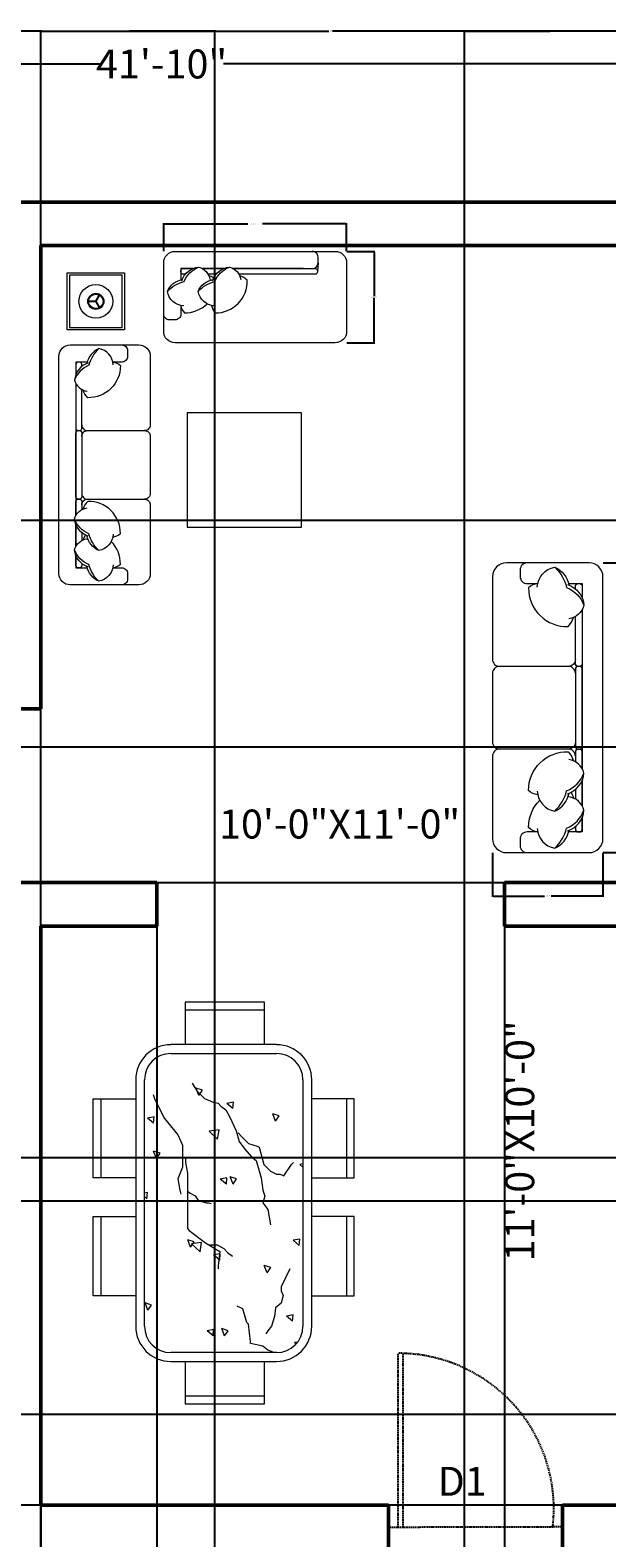
# Model space of a CAD drawing. Units: inches. Extents: x 3 to 576, y -689 to 51.
# Tile 18 of 21: x 262 to 381, y -261 to 51. Entities that reach past the tile are written whole.
import ezdxf

# ---------------------------------------------------------------- set-up
doc = ezdxf.new("R2010")
doc.units = ezdxf.units.IN
doc.header["$MEASUREMENT"] = 0
doc.linetypes.add('DASHED2', pattern=[0.375, 0.25, -0.125])
for name, color, linetype, lineweight in [('A-ANNO-DIMS', 2, 'Continuous', 18), ('A-ANNO-TEXT', 3, 'Continuous', 18), ('A-AREA-IDEN', 7, 'Continuous', 18), ('A-DOOR', 4, 'DASHED2', 25), ('A-FURN', 8, 'Continuous', 18), ('A-WALL', 7, 'Continuous', 50)]:
    doc.layers.add(name, color=color, linetype=linetype, lineweight=lineweight)
doc.styles.get("Standard").update_dxf_attribs({"font": 'arial.ttf'})
doc.dimstyles.get("Standard").update_dxf_attribs({"dimtxt": 0.18, "dimasz": 0.18, "dimexe": 0.18, "dimexo": 0.0625, "dimgap": 0.09, "dimtad": 0, "dimtih": 1, "dimtoh": 1, "dimdec": 0, "dimzin": 0, "dimdsep": 46, "dimlunit": 3, "dimtxsty": 'Standard', "dimcen": 0.09, "dimadec": 0, "dimazin": 0, "dimtfac": 1, "dimtdec": 0, "dimtofl": 0, "dimtmove": 0, "dimatfit": 3, "dimfxl": 1, "dimtolj": 1, "dimtzin": 0, "dimarcsym": 0})

# ---------------------------------------------------------------- blocks, each defined once
blk = doc.blocks.new('*D1')
at = {"layer": 'A-ANNO-DIMS', "color": 0, "lineweight": -2, "transparency": 16777216}
for p, q in [((38.29, 15.75), (38.29, 44.49)), ((38.47, 44.31), (276.45, 44.31)), ((540.11, 44.31), (302.14, 44.31)), ((540.29, 15.75), (540.29, 44.49))]:
    blk.add_line(p, q, dxfattribs=at)
at = {"layer": 'A-ANNO-DIMS', "color": 0, "transparency": 16777216}
for points in [[(38.47, 44.34), (38.47, 44.28), (38.29, 44.31)], [(540.11, 44.34), (540.11, 44.28), (540.29, 44.31)]]:
    blk.add_solid(points, dxfattribs=at)
at = {"layer": 'Defpoints', "color": 0, "transparency": 16777216}
for p in [(540.29, 44.31), (38.29, 15.69), (540.29, 15.69)]:
    blk.add_point(p, dxfattribs=at)
at = {"layer": 'A-ANNO-DIMS', "color": 0, "transparency": 16777216, "insert": (289.29, 44.31), "char_height": 6, "attachment_point": 5}
blk.add_mtext('\\A1;41\'-10"', dxfattribs=at)
blk = doc.blocks.new('DAY BED1')
at = {"color": 0}
blk.add_line((0.3, 0.25), (0.225, 0.255), dxfattribs=at)
blk.add_lwpolyline([(-0.3, 0, -0.414214), (-0.4, 0.1), (-0.4, 0.1, 0.317837), (-0.4, 0.1, -0.414214), (-0.4, 0.1), (-0.4, 0.1, 1.186185), (-0.4, 0.1, -0.414214), (-0.4, 0.1), (-0.4, 1.5, -0.414214), (-0.3, 1.6), (0.3, 1.6, -0.414214), (0.4, 1.5), (0.4, 0.1, -0.414214), (0.3, 0)], format="xyb", close=True, dxfattribs=at)
for points in [[(-0.073, 1.45), (-0.15, 1.45, -0.414214), (-0.2, 1.5), (-0.2, 1.55, -0.414214), (-0.15, 1.6)], [(-0.076, 1.425, -0.356772), (0.05, 1.568, -0.249542), (0.154, 1.438, 9.61688)], [(0.05, 1.568, -0.14773), (0.136, 1.422, -0.213343), (0.262, 1.293, -0.178662)], [(-0.073, 1.45, 0.165541), (-0.139, 1.419, 0.200231), (-0.058, 1.221, 0.121523)], [(0.143, 1.442, -0.306663), (0.262, 1.293, -0.30633), (0.154, 1.196, 0.872847)], [(0.25, 1.345), (0.25, 1.45), (0.152, 1.45, -0.414214)], [(0.2, 1.412), (0.2, 1.43, -0.414214), (0.22, 1.45), (0.23, 1.45, -0.414214), (0.25, 1.43)], [(0.25, 1.43), (0.25, 1.345, -0.414214)], [(-0.076, 1.156, -0.356772), (0.05, 1.299, -0.249542), (0.154, 1.169, 9.61688)], [(0.05, 1.299, -0.14773), (0.136, 1.153, -0.213343), (0.262, 1.024, -0.178662)], [(0.168, 1.163, 0.071865), (0.187, 1.205, -7.115464)], [(0.2, 1.142), (0.2, 1.211, -0.414214)], [(0.25, 1.262), (0.25, 1.075, -0.414214)], [(-0.073, 1.181, 0.165541), (-0.139, 1.15, 0.425989), (0.148, 0.869, 0.121523), (0.187, 0.936, -7.115464)], [(0.143, 1.173, -0.306663), (0.262, 1.024, -0.30633), (0.154, 0.926, 0.872847)], [(0.25, 0.992), (0.25, 0.275, -0.414214), (0.23, 0.255), (0.22, 0.255, -0.414214), (0.2, 0.275), (0.2, 0.942, -0.414214)], [(0.25, 0.377), (0.25, 0.3, 0.414214), (0.3, 0.25), (0.35, 0.25, 0.414214), (0.4, 0.3)]]:
    blk.add_lwpolyline(points, format="xyb", dxfattribs=at)
for points in [[(0.25, 1.075), (0.25, 1.262)], [(0.25, 0.377), (0.25, 0.992)]]:
    blk.add_lwpolyline(points, dxfattribs=at)
blk = doc.blocks.new('DINING-SET-6')
for p, q in [((35.44, 83.21), (19.03, 83.21)), ((19.03, 83.21), (19.03, 74.43)), ((19.03, 81.61), (35.44, 81.61)), ((35.44, 74.43), (35.44, 83.21)), ((37.96, 74.43), (16.08, 74.43)), ((16.08, 72.6), (37.96, 72.6)), ((8.79, 67.13), (8.79, 16.08)), ((10.61, 16.08), (10.61, 67.13)), ((20.49, 66.46), (21.48, 64.87)), ((43.43, 67.13), (43.43, 16.08)), ((45.25, 16.08), (45.25, 67.13)), ((0, 46.82), (0, 63.23)), ((0, 63.23), (8.79, 63.23)), ((1.6, 63.23), (1.6, 46.82)), ((12.38, 64.08), (12.77, 63.09)), ((12.77, 63.09), (14.75, 59.12)), ((21.9, 63.9), (21.31, 65.43)), ((22.64, 64.98), (21.31, 65.43)), ((21.48, 64.87), (23.07, 63.29)), ((21.9, 63.9), (22.63, 64.98)), ((23.07, 63.29), (24.85, 62.49)), ((24.85, 62.49), (25.84, 62.3)), ((29.06, 62.49), (27.69, 62.24)), ((28.94, 61.18), (29.06, 62.49)), ((54.04, 63.23), (45.25, 63.23)), ((52.44, 63.23), (52.44, 46.82)), ((54.04, 46.82), (54.04, 63.23)), ((12.6, 59.46), (11.23, 59.2)), ((12.49, 58.15), (12.6, 59.46)), ((25.84, 62.3), (26.44, 61.7)), ((26.44, 61.7), (27.43, 60.91)), ((27.43, 60.91), (28.22, 59.52)), ((28.94, 61.18), (27.69, 62.24)), ((28.22, 59.52), (29.6, 56.55)), ((38.5, 59.66), (37.18, 60.1)), ((37.77, 58.57), (37.18, 60.1)), ((37.77, 58.57), (38.5, 59.66)), ((12.49, 58.15), (11.23, 59.2)), ((14.75, 59.12), (17.52, 55.75)), ((26.06, 56.77), (23.98, 56.52)), ((25.76, 54.82), (23.98, 56.52)), ((25.76, 54.82), (26.06, 56.77)), ((29.6, 56.55), (30.2, 54.36)), ((17.52, 55.75), (18.51, 53.57)), ((18.51, 53.57), (18.51, 49.01)), ((30, 56.15), (30.79, 55.36)), ((30.2, 54.36), (31.39, 52.78)), ((30.79, 55.36), (32.18, 53.97)), ((32.18, 53.97), (33.96, 53.37)), ((33.96, 53.37), (34.36, 53.18)), ((34.36, 53.18), (35.35, 49.61)), ((13.09, 50.84), (12.5, 52.37)), ((13.83, 51.93), (12.5, 52.37)), ((13.09, 50.84), (13.83, 51.92)), ((19.11, 51.19), (19.11, 50)), ((19.11, 50), (19.5, 47.82)), ((31.39, 52.78), (32.77, 51.19)), ((32.77, 51.19), (33.76, 50.4)), ((33.76, 50.4), (34.75, 46.83)), ((41.09, 49.61), (41.49, 50)), ((18.51, 49.01), (17.52, 46.63)), ((19.5, 47.82), (19.5, 36.32)), ((28.96, 45.51), (28.37, 47.05)), ((29.69, 46.6), (28.37, 47.05)), ((35.35, 49.61), (36.73, 48.22)), ((36.73, 48.22), (37.92, 47.62)), ((37.92, 47.62), (38.71, 47.62)), ((38.71, 47.62), (39.5, 47.23)), ((39.5, 47.23), (41.09, 49.61)), ((43.43, 49.7), (42.77, 49.58)), ((43.43, 49.03), (42.77, 49.58)), ((8.79, 46.82), (0, 46.82)), ((11.23, 43.76), (10.61, 43.65)), ((11.11, 42.46), (11.23, 43.76)), ((17.52, 46.63), (17.92, 44.25)), ((17.92, 44.25), (18.12, 43.46)), ((19.5, 44.06), (20.09, 43.66)), ((27.69, 46.8), (26.31, 46.55)), ((27.57, 45.49), (26.31, 46.55)), ((27.57, 45.49), (27.68, 46.8)), ((28.96, 45.51), (29.69, 46.6)), ((34.75, 46.83), (35.15, 44.25)), ((35.15, 44.25), (35.54, 43.06)), ((45.25, 46.82), (54.04, 46.82)), ((11.11, 42.46), (10.61, 42.88)), ((20.09, 43.66), (21.08, 43.07)), ((21.08, 43.07), (21.68, 42.27)), ((21.68, 42.27), (22.67, 41.88)), ((22.67, 41.88), (23.46, 41.68)), ((23.46, 41.68), (23.85, 41.68)), ((23.85, 41.68), (24.45, 41.48)), ((35.54, 43.06), (35.15, 41.68)), ((35.15, 41.68), (36.14, 40.29)), ((0, 22.39), (0, 38.8)), ((0, 38.8), (8.79, 38.8)), ((1.6, 38.8), (1.6, 22.39)), ((36.14, 40.29), (36.73, 37.12)), ((54.04, 38.8), (45.25, 38.8)), ((52.44, 38.8), (52.44, 22.39)), ((54.04, 22.39), (54.04, 38.8)), ((19.5, 36.32), (19.9, 35.93)), ((19.9, 35.93), (23.27, 33.35)), ((20.15, 32.45), (19.56, 33.99)), ((20.88, 33.54), (19.56, 33.99)), ((20.15, 32.45), (20.88, 33.54)), ((22.44, 33.42), (20.36, 33.17)), ((22.14, 31.47), (20.36, 33.17)), ((22.14, 31.47), (22.44, 33.42)), ((23.27, 33.35), (26.24, 31.57)), ((23.86, 32.95), (25.64, 32.95)), ((25.64, 32.95), (27.03, 32.16)), ((26.24, 31.57), (25.84, 28.59)), ((27.03, 32.16), (27.82, 31.37)), ((27.82, 31.37), (28.81, 30.57)), ((42.77, 34.14), (41.4, 33.89)), ((42.65, 32.83), (41.4, 33.89)), ((42.65, 32.83), (42.77, 34.14)), ((26.31, 31.11), (24.94, 30.85)), ((26.2, 29.8), (24.94, 30.85)), ((25.84, 28.59), (25.84, 28)), ((26.2, 29.8), (26.31, 31.11)), ((36.01, 27.13), (35.43, 28.66)), ((36.75, 28.22), (35.43, 28.66)), ((36.01, 27.13), (36.75, 28.22)), ((40.69, 28), (38.9, 24.23)), ((8.79, 22.39), (0, 22.39)), ((38.9, 24.23), (38.9, 23.44)), ((38.9, 23.44), (39.3, 22.45)), ((39.3, 22.45), (38.9, 20.86)), ((45.25, 22.39), (54.04, 22.39)), ((11.34, 19.39), (10.75, 20.93)), ((12.07, 20.48), (10.75, 20.93)), ((11.34, 19.39), (12.07, 20.48)), ((30.99, 19.67), (29.8, 20.27)), ((31.78, 16.89), (30.99, 19.67)), ((37.72, 19.87), (37.52, 18.09)), ((38.9, 20.86), (37.72, 19.87)), ((32.18, 16.5), (31.78, 16.89)), ((32.57, 12.93), (32.18, 16.5)), ((36.92, 16.1), (36.13, 15.11)), ((37.52, 18.09), (36.92, 16.1)), ((41.28, 17.14), (40.02, 18.2)), ((41.4, 18.45), (40.03, 18.2)), ((41.28, 17.14), (41.4, 18.45)), ((24.94, 15.41), (23.57, 15.16)), ((24.82, 14.11), (23.57, 15.16)), ((24.82, 14.11), (24.94, 15.41)), ((27.21, 14.07), (26.62, 15.6)), ((27.94, 15.16), (26.62, 15.6)), ((27.21, 14.07), (27.94, 15.16)), ((32.57, 12.53), (32.57, 12.93)), ((35.15, 11.94), (32.57, 12.53)), ((36.13, 15.11), (35.74, 14.52)), ((42.34, 12.8), (41.67, 12.72)), ((42.01, 12.4), (41.67, 12.72)), ((37.96, 10.61), (16.08, 10.61)), ((36.14, 11.15), (35.15, 11.94)), ((37.13, 10.75), (36.14, 11.15)), ((16.08, 8.79), (37.96, 8.79)), ((19.03, 8.79), (19.03, 0)), ((35.44, 0), (35.44, 8.79)), ((35.44, 1.6), (19.03, 1.6)), ((19.03, 0), (35.44, 0))]:
    blk.add_line(p, q)
for centre, radius, start, end in [((16.08, 67.13), 7.29, 90, 180), ((16.08, 67.13), 5.47, 90, 180), ((37.96, 67.13), 7.29, 0, 90), ((37.96, 67.13), 5.47, 0, 90), ((16.08, 16.08), 7.29, 180, 270), ((16.08, 16.08), 5.47, 180, 270), ((37.96, 16.08), 5.47, 270, 0), ((37.96, 16.08), 7.29, 270, 0)]:
    blk.add_arc(centre, radius, start, end)
blk = doc.blocks.new('SOFA-3SEAT')
at = {"ltscale": 0.03}
blk.add_lwpolyline([(2.86, 60.03, 0.414214), (0, 57.17), (0, 40.02, 0.414214), (1.43, 38.59, 0.414214), (0, 37.16), (0, 22.87, 0.414214), (1.43, 21.44, 0.414214), (0, 20.01), (0, 2.86, 0.414214), (2.86, 0), (20.01, 0, 0.414214), (22.87, 2.86), (22.87, 57.17, 0.414214), (20.01, 60.03)], format="xyb", close=True, dxfattribs=at)
for points in [[(7.15, 60.03, 0.414214), (5.72, 58.6), (5.72, 57.17, 0.414214), (7.15, 55.74), (9.36, 55.74)], [(9.27, 55.02, -0.356772), (12.88, 59.12, -0.249542), (15.84, 55.41, 9.61688)], [(12.88, 59.12, -0.14773), (15.33, 54.94, -0.213343), (18.93, 51.25, -0.178662)], [(9.36, 55.74, 0.165541), (7.47, 54.86, 0.425989), (15.66, 46.83, 0.121523), (16.79, 48.74, -7.115464)], [(15.53, 55.52, -0.306663), (18.93, 51.25, -0.30633), (15.82, 48.47, 0.872847)], [(17.15, 54.65), (17.15, 55.17, -0.414214), (17.72, 55.74), (18.01, 55.74, -0.414214), (18.58, 55.17)], [(18.58, 55.17), (18.58, 52.73, -0.414214)], [(18.58, 50.35), (18.58, 39.16, -0.414214), (18.01, 38.59), (17.72, 38.59, -0.414214), (17.15, 39.16), (17.15, 48.91, -0.414214)], [(17.15, 40.02, -0.414214), (15.72, 38.59), (1.43, 38.59, -0.414214)], [(17.15, 37.16, 0.414214), (15.72, 38.59)], [(17.15, 22.87, -0.414214), (15.72, 21.44)], [(17.15, 20.01, 0.414214), (15.72, 21.44), (1.43, 21.44, 0.414214)], [(9.36, 11.98, -0.165541), (7.47, 12.87, -0.425989), (15.66, 20.89, -0.121523), (16.79, 18.99, 7.115464)], [(15.53, 12.21, 0.306663), (18.93, 16.47, 0.30633), (15.82, 19.26, -0.872847)], [(18.58, 17.37), (18.58, 20.87, 0.414214), (18.01, 21.44), (17.72, 21.44, 0.414214), (17.15, 20.87), (17.15, 18.81, 0.414214)], [(12.88, 8.61, 0.14773), (15.33, 12.79, 0.213343), (18.93, 16.47, 0.178662)], [(9.27, 12.7, 0.356772), (12.88, 8.61, 0.249542), (15.84, 12.32, -9.61688)], [(17.15, 13.08), (17.15, 11.11, 0.414214)], [(18.58, 9.67), (18.58, 14.99, 0.414214)], [(9.36, 4.28, -0.165541), (7.47, 5.17, -0.200231), (9.77, 10.84, -0.121523)], [(15.53, 4.51, 0.306663), (18.93, 8.77, 0.30633), (15.82, 11.56, -0.872847)], [(16.23, 12.49, -0.071865), (16.79, 11.29, 7.115464)], [(12.88, 0.91, 0.14773), (15.33, 5.09, 0.213343), (18.93, 8.77, 0.178662)], [(18.58, 7.29), (18.58, 4.29), (15.77, 4.29, 0.414214)], [(18.58, 4.86), (18.58, 7.29, 0.414214)], [(9.36, 4.29), (7.15, 4.29, 0.414214), (5.72, 2.86), (5.72, 1.43, 0.414214), (7.15, 0)], [(9.27, 5, 0.356772), (12.88, 0.91, 0.249542), (15.84, 4.62, -9.61688)], [(17.15, 5.38), (17.15, 4.86, 0.414214), (17.72, 4.29), (18.01, 4.29, 0.414214), (18.58, 4.86)]]:
    blk.add_lwpolyline(points, format="xyb")
for points in [[(15.77, 55.74), (18.58, 55.74), (18.58, 52.73)], [(18.58, 50.35), (18.58, 17.37)], [(18.58, 14.99), (18.58, 9.67)]]:
    blk.add_lwpolyline(points)
blk.add_lwpolyline([(18.58, 22.01), (18.58, 38.02, 0.414214), (18.01, 38.59), (17.72, 38.59, 0.414214), (17.15, 38.02), (17.15, 22.01, 0.414214), (17.72, 21.44), (18.01, 21.44, 0.414214)], format="xyb", close=True)
blk = doc.blocks.new('DOOR-SWING-900')
for p, q in [((35.95, 36), (35.95, 34)), ((36, 2), (35.95, 34)), ((36, 2), (0, 2)), ((36, 0), (36, 2))]:
    blk.add_line(p, q)
blk.add_arc((32.22, 2), 32.22, 83.347, 180)
blk = doc.blocks.new('*D31')
at = {"layer": 'A-ANNO-DIMS', "color": 0, "lineweight": -2, "transparency": 16777216}
for p, q in [((289.72, 5.54), (289.72, 11.34)), ((289.9, 11.16), (307.16, 11.16)), ((327.42, 11.16), (310.15, 11.16)), ((327.6, 5.54), (327.6, 11.34))]:
    blk.add_line(p, q, dxfattribs=at)
at = {"layer": 'A-ANNO-DIMS', "color": 0, "transparency": 16777216}
for points in [[(289.9, 11.19), (289.9, 11.13), (289.72, 11.16)], [(327.42, 11.19), (327.42, 11.13), (327.6, 11.16)]]:
    blk.add_solid(points, dxfattribs=at)
at = {"layer": 'Defpoints', "color": 0, "transparency": 16777216}
for p in [(289.72, 11.16), (289.72, 5.48), (327.6, 5.48)]:
    blk.add_point(p, dxfattribs=at)
at = {"layer": 'A-ANNO-DIMS', "color": 0, "transparency": 16777216, "insert": (308.66, 11.16), "char_height": 0.18, "attachment_point": 5}
blk.add_mtext('\\A1;2-SEAT SOFA 3\'-2" TYP.', dxfattribs=at)
blk = doc.blocks.new('*D32')
at = {"layer": 'A-ANNO-DIMS', "color": 0, "lineweight": -2, "transparency": 16777216}
for p, q in [((327.66, 5.48), (333.46, 5.48)), ((333.28, 5.3), (333.28, -3.81)), ((333.28, -13.28), (333.28, -4.17)), ((327.66, -13.46), (333.46, -13.46))]:
    blk.add_line(p, q, dxfattribs=at)
at = {"layer": 'A-ANNO-DIMS', "color": 0, "transparency": 16777216}
for points in [[(333.25, 5.3), (333.31, 5.3), (333.28, 5.48)], [(333.25, -13.28), (333.31, -13.28), (333.28, -13.46)]]:
    blk.add_solid(points, dxfattribs=at)
at = {"layer": 'Defpoints', "color": 0, "transparency": 16777216}
for p in [(327.6, 5.48), (333.28, 5.48), (327.6, -13.46)]:
    blk.add_point(p, dxfattribs=at)
at = {"layer": 'A-ANNO-DIMS', "color": 0, "transparency": 16777216, "insert": (333.28, -3.99), "char_height": 0.18, "attachment_point": 5}
blk.add_mtext('\\A1;1\'-7" TYP.', dxfattribs=at)
blk = doc.blocks.new('*D35')
at = {"layer": 'A-ANNO-DIMS', "color": 0, "lineweight": -2, "transparency": 16777216}
for p, q in [((380.75, -59.06), (389.87, -59.06)), ((389.69, -59.24), (389.69, -88.89)), ((389.69, -118.91), (389.69, -89.26)), ((380.75, -119.09), (389.87, -119.09))]:
    blk.add_line(p, q, dxfattribs=at)
at = {"layer": 'A-ANNO-DIMS', "color": 0, "transparency": 16777216}
for points in [[(389.66, -59.24), (389.72, -59.24), (389.69, -59.06)], [(389.66, -118.91), (389.72, -118.91), (389.69, -119.09)]]:
    blk.add_solid(points, dxfattribs=at)
at = {"layer": 'Defpoints', "color": 0, "transparency": 16777216}
for p in [(380.69, -59.06), (389.69, -59.06), (380.69, -119.09)]:
    blk.add_point(p, dxfattribs=at)
at = {"layer": 'A-ANNO-DIMS', "color": 0, "transparency": 16777216, "insert": (389.69, -89.08), "char_height": 0.18, "attachment_point": 5}
blk.add_mtext('\\A1;3-SEAT SOFA 5\'-0" TYP.', dxfattribs=at)
blk = doc.blocks.new('*D36')
at = {"layer": 'A-ANNO-DIMS', "color": 0, "lineweight": -2, "transparency": 16777216}
for p, q in [((357.82, -119.15), (357.82, -128.27)), ((380.69, -119.15), (380.69, -128.27)), ((358, -128.09), (368.55, -128.09)), ((380.51, -128.09), (369.95, -128.09))]:
    blk.add_line(p, q, dxfattribs=at)
at = {"layer": 'A-ANNO-DIMS', "color": 0, "transparency": 16777216}
for points in [[(358, -128.06), (358, -128.12), (357.82, -128.09)], [(380.51, -128.06), (380.51, -128.12), (380.69, -128.09)]]:
    blk.add_solid(points, dxfattribs=at)
at = {"layer": 'Defpoints', "color": 0, "transparency": 16777216}
for p in [(357.82, -119.09), (380.69, -119.09), (380.69, -128.09)]:
    blk.add_point(p, dxfattribs=at)
at = {"layer": 'A-ANNO-DIMS', "color": 0, "transparency": 16777216, "insert": (369.25, -128.09), "char_height": 0.18, "attachment_point": 5}
blk.add_mtext('\\A1;1\'-11" TYP.', dxfattribs=at)
blk = doc.blocks.new('*D43')
at = {"layer": 'A-ANNO-DIMS', "color": 0, "lineweight": -2, "transparency": 16777216}
for p, q in [((255.29, 6.75), (255.29, 51.32)), ((255.47, 51.14), (259.46, 51.14)), ((264.11, 51.14), (260.12, 51.14)), ((264.29, 6.75), (264.29, 51.32))]:
    blk.add_line(p, q, dxfattribs=at)
at = {"layer": 'A-ANNO-DIMS', "color": 0, "transparency": 16777216}
for points in [[(255.47, 51.17), (255.47, 51.11), (255.29, 51.14)], [(264.11, 51.17), (264.11, 51.11), (264.29, 51.14)]]:
    blk.add_solid(points, dxfattribs=at)
at = {"layer": 'Defpoints', "color": 0, "transparency": 16777216}
for p in [(264.29, 51.14), (255.29, 6.69), (264.29, 6.69)]:
    blk.add_point(p, dxfattribs=at)
at = {"layer": 'A-ANNO-DIMS', "color": 0, "transparency": 16777216, "insert": (259.79, 51.14), "char_height": 0.18, "attachment_point": 5}
blk.add_mtext('\\A1;0\'-9"', dxfattribs=at)
blk = doc.blocks.new('*D44')
at = {"layer": 'A-ANNO-DIMS', "color": 0, "lineweight": -2, "transparency": 16777216}
for p, q in [((264.29, 6.75), (264.29, 51.32)), ((264.47, 51.14), (323.9, 51.14)), ((384.11, 51.14), (324.68, 51.14)), ((384.29, 6.75), (384.29, 51.32))]:
    blk.add_line(p, q, dxfattribs=at)
at = {"layer": 'A-ANNO-DIMS', "color": 0, "transparency": 16777216}
for points in [[(264.47, 51.17), (264.47, 51.11), (264.29, 51.14)], [(384.11, 51.17), (384.11, 51.11), (384.29, 51.14)]]:
    blk.add_solid(points, dxfattribs=at)
at = {"layer": 'Defpoints', "color": 0, "transparency": 16777216}
for p in [(384.29, 51.14), (264.29, 6.69), (384.29, 6.69)]:
    blk.add_point(p, dxfattribs=at)
at = {"layer": 'A-ANNO-DIMS', "color": 0, "transparency": 16777216, "insert": (324.29, 51.14), "char_height": 0.18, "attachment_point": 5}
blk.add_mtext('\\A1;10\'-0"', dxfattribs=at)
blk = doc.blocks.new('*D64')
at = {"layer": 'A-ANNO-DIMS', "color": 0, "lineweight": -2, "transparency": 16777216}
for p, q in [((540.23, 15.69), (2.66, 15.69)), ((2.84, 15.51), (2.84, -17.13)), ((2.84, -50.13), (2.84, -17.49)), ((531.23, -50.31), (2.66, -50.31))]:
    blk.add_line(p, q, dxfattribs=at)
at = {"layer": 'A-ANNO-DIMS', "color": 0, "transparency": 16777216}
for points in [[(2.81, 15.51), (2.87, 15.51), (2.84, 15.69)], [(2.81, -50.13), (2.87, -50.13), (2.84, -50.31)]]:
    blk.add_solid(points, dxfattribs=at)
at = {"layer": 'Defpoints', "color": 0, "transparency": 16777216}
for p in [(540.29, 15.69), (2.84, -50.31), (531.29, -50.31)]:
    blk.add_point(p, dxfattribs=at)
at = {"layer": 'A-ANNO-DIMS', "color": 0, "transparency": 16777216, "insert": (2.84, -17.31), "char_height": 0.18, "attachment_point": 5}
blk.add_mtext('\\A1;5\'-6"', dxfattribs=at)
blk = doc.blocks.new('*D65')
at = {"layer": 'A-ANNO-DIMS', "color": 0, "lineweight": -2, "transparency": 16777216}
for p, q in [((531.23, -50.31), (2.66, -50.31)), ((2.84, -50.49), (2.84, -116.13)), ((2.84, -182.13), (2.84, -116.49)), ((531.23, -182.31), (2.66, -182.31))]:
    blk.add_line(p, q, dxfattribs=at)
at = {"layer": 'A-ANNO-DIMS', "color": 0, "transparency": 16777216}
for points in [[(2.81, -50.49), (2.87, -50.49), (2.84, -50.31)], [(2.81, -182.13), (2.87, -182.13), (2.84, -182.31)]]:
    blk.add_solid(points, dxfattribs=at)
at = {"layer": 'Defpoints', "color": 0, "transparency": 16777216}
for p in [(531.29, -50.31), (2.84, -182.31), (531.29, -182.31)]:
    blk.add_point(p, dxfattribs=at)
at = {"layer": 'A-ANNO-DIMS', "color": 0, "transparency": 16777216, "insert": (2.84, -116.31), "char_height": 0.18, "attachment_point": 5}
blk.add_mtext('\\A1;11\'-0"', dxfattribs=at)
blk = doc.blocks.new('*D66')
at = {"layer": 'A-ANNO-DIMS', "color": 0, "lineweight": -2, "transparency": 16777216}
for p, q in [((531.23, -182.31), (2.66, -182.31)), ((2.84, -182.49), (2.84, -186.63)), ((2.84, -191.13), (2.84, -186.99)), ((531.23, -191.31), (2.66, -191.31))]:
    blk.add_line(p, q, dxfattribs=at)
at = {"layer": 'A-ANNO-DIMS', "color": 0, "transparency": 16777216}
for points in [[(2.81, -182.49), (2.87, -182.49), (2.84, -182.31)], [(2.81, -191.13), (2.87, -191.13), (2.84, -191.31)]]:
    blk.add_solid(points, dxfattribs=at)
at = {"layer": 'Defpoints', "color": 0, "transparency": 16777216}
for p in [(531.29, -182.31), (2.84, -191.31), (531.29, -191.31)]:
    blk.add_point(p, dxfattribs=at)
at = {"layer": 'A-ANNO-DIMS', "color": 0, "transparency": 16777216, "insert": (2.84, -186.81), "char_height": 0.18, "attachment_point": 5}
blk.add_mtext('\\A1;0\'-9"', dxfattribs=at)
blk = doc.blocks.new('*D67')
at = {"layer": 'A-ANNO-DIMS', "color": 0, "lineweight": -2, "transparency": 16777216}
for p, q in [((531.23, -191.31), (2.66, -191.31)), ((2.84, -191.49), (2.84, -222.63)), ((2.84, -254.13), (2.84, -222.99)), ((531.23, -254.31), (2.66, -254.31))]:
    blk.add_line(p, q, dxfattribs=at)
at = {"layer": 'A-ANNO-DIMS', "color": 0, "transparency": 16777216}
for points in [[(2.81, -191.49), (2.87, -191.49), (2.84, -191.31)], [(2.81, -254.13), (2.87, -254.13), (2.84, -254.31)]]:
    blk.add_solid(points, dxfattribs=at)
at = {"layer": 'Defpoints', "color": 0, "transparency": 16777216}
for p in [(531.29, -191.31), (2.84, -254.31), (531.29, -254.31)]:
    blk.add_point(p, dxfattribs=at)
at = {"layer": 'A-ANNO-DIMS', "color": 0, "transparency": 16777216, "insert": (2.84, -222.81), "char_height": 0.18, "attachment_point": 5}
blk.add_mtext('\\A1;5\'-3"', dxfattribs=at)
blk = doc.blocks.new('*D68')
at = {"layer": 'A-ANNO-DIMS', "color": 0, "lineweight": -2, "transparency": 16777216}
for p, q in [((531.23, -254.31), (2.66, -254.31)), ((2.84, -254.49), (2.84, -258.63)), ((2.84, -263.13), (2.84, -258.99)), ((531.23, -263.31), (2.66, -263.31))]:
    blk.add_line(p, q, dxfattribs=at)
at = {"layer": 'A-ANNO-DIMS', "color": 0, "transparency": 16777216}
for points in [[(2.81, -254.49), (2.87, -254.49), (2.84, -254.31)], [(2.81, -263.13), (2.87, -263.13), (2.84, -263.31)]]:
    blk.add_solid(points, dxfattribs=at)
at = {"layer": 'Defpoints', "color": 0, "transparency": 16777216}
for p in [(531.29, -254.31), (2.84, -263.31), (531.29, -263.31)]:
    blk.add_point(p, dxfattribs=at)
at = {"layer": 'A-ANNO-DIMS', "color": 0, "transparency": 16777216, "insert": (2.84, -258.81), "char_height": 0.18, "attachment_point": 5}
blk.add_mtext('\\A1;0\'-9"', dxfattribs=at)
blk = doc.blocks.new('*D87')
at = {"layer": 'A-ANNO-DIMS', "color": 0, "lineweight": -2, "transparency": 16777216}
for p, q in [((195.85, -97.15), (575.92, -97.15)), ((575.74, -97.33), (575.74, -111.05)), ((575.74, -125.13), (575.74, -111.41)), ((195.85, -125.31), (575.92, -125.31))]:
    blk.add_line(p, q, dxfattribs=at)
at = {"layer": 'A-ANNO-DIMS', "color": 0, "transparency": 16777216}
for points in [[(575.71, -97.33), (575.77, -97.33), (575.74, -97.15)], [(575.71, -125.13), (575.77, -125.13), (575.74, -125.31)]]:
    blk.add_solid(points, dxfattribs=at)
at = {"layer": 'Defpoints', "color": 0, "transparency": 16777216}
for p in [(195.78, -97.15), (575.74, -97.15), (195.78, -125.31)]:
    blk.add_point(p, dxfattribs=at)
at = {"layer": 'A-ANNO-DIMS', "color": 0, "transparency": 16777216, "insert": (575.74, -111.23), "char_height": 0.18, "attachment_point": 5}
blk.add_mtext('\\A1;2\'-4"', dxfattribs=at)
blk = doc.blocks.new('*D115')
at = {"layer": 'A-ANNO-DIMS', "color": 0, "lineweight": -2, "transparency": 16777216}
for p, q in [((264.29, -134.37), (264.29, -688.94)), ((288.29, -134.37), (288.29, -688.94)), ((264.47, -688.76), (275.96, -688.76)), ((288.11, -688.76), (276.62, -688.76))]:
    blk.add_line(p, q, dxfattribs=at)
at = {"layer": 'A-ANNO-DIMS', "color": 0, "transparency": 16777216}
for points in [[(264.47, -688.73), (264.47, -688.79), (264.29, -688.76)], [(288.11, -688.73), (288.11, -688.79), (288.29, -688.76)]]:
    blk.add_solid(points, dxfattribs=at)
at = {"layer": 'Defpoints', "color": 0, "transparency": 16777216}
for p in [(264.29, -134.31), (288.29, -134.31), (288.29, -688.76)]:
    blk.add_point(p, dxfattribs=at)
at = {"layer": 'A-ANNO-DIMS', "color": 0, "transparency": 16777216, "insert": (276.29, -688.76), "char_height": 0.18, "attachment_point": 5}
blk.add_mtext('\\A1;2\'-0"', dxfattribs=at)
blk = doc.blocks.new('*D116')
at = {"layer": 'A-ANNO-DIMS', "color": 0, "lineweight": -2, "transparency": 16777216}
for p, q in [((360.29, -134.37), (360.29, -688.94)), ((384.29, -134.37), (384.29, -688.94)), ((360.47, -688.76), (371.96, -688.76)), ((384.11, -688.76), (372.62, -688.76))]:
    blk.add_line(p, q, dxfattribs=at)
at = {"layer": 'A-ANNO-DIMS', "color": 0, "transparency": 16777216}
for points in [[(360.47, -688.73), (360.47, -688.79), (360.29, -688.76)], [(384.11, -688.73), (384.11, -688.79), (384.29, -688.76)]]:
    blk.add_solid(points, dxfattribs=at)
at = {"layer": 'Defpoints', "color": 0, "transparency": 16777216}
for p in [(360.29, -134.31), (384.29, -134.31), (384.29, -688.76)]:
    blk.add_point(p, dxfattribs=at)
at = {"layer": 'A-ANNO-DIMS', "color": 0, "transparency": 16777216, "insert": (372.29, -688.76), "char_height": 0.18, "attachment_point": 5}
blk.add_mtext('\\A1;2\'-0"', dxfattribs=at)
blk = doc.blocks.new('*D117')
at = {"layer": 'A-ANNO-DIMS', "color": 0, "lineweight": -2, "transparency": 16777216}
for p, q in [((264.29, -506.25), (264.29, 51.32)), ((264.47, 51.14), (281.96, 51.14)), ((300.11, 51.14), (282.62, 51.14)), ((300.29, -506.25), (300.29, 51.32))]:
    blk.add_line(p, q, dxfattribs=at)
at = {"layer": 'A-ANNO-DIMS', "color": 0, "transparency": 16777216}
for points in [[(264.47, 51.17), (264.47, 51.11), (264.29, 51.14)], [(300.11, 51.17), (300.11, 51.11), (300.29, 51.14)]]:
    blk.add_solid(points, dxfattribs=at)
at = {"layer": 'Defpoints', "color": 0, "transparency": 16777216}
for p in [(300.29, 51.14), (264.29, -506.31), (300.29, -506.31)]:
    blk.add_point(p, dxfattribs=at)
at = {"layer": 'A-ANNO-DIMS', "color": 0, "transparency": 16777216, "insert": (282.29, 51.14), "char_height": 0.18, "attachment_point": 5}
blk.add_mtext('\\A1;3\'-0"', dxfattribs=at)
blk = doc.blocks.new('*D118')
at = {"layer": 'A-ANNO-DIMS', "color": 0, "lineweight": -2, "transparency": 16777216}
for p, q in [((352.02, -506.25), (352.02, 51.32)), ((352.2, 51.14), (369.69, 51.14)), ((387.84, 51.14), (370.35, 51.14)), ((388.02, -506.25), (388.02, 51.32))]:
    blk.add_line(p, q, dxfattribs=at)
at = {"layer": 'A-ANNO-DIMS', "color": 0, "transparency": 16777216}
for points in [[(352.2, 51.17), (352.2, 51.11), (352.02, 51.14)], [(387.84, 51.17), (387.84, 51.11), (388.02, 51.14)]]:
    blk.add_solid(points, dxfattribs=at)
at = {"layer": 'Defpoints', "color": 0, "transparency": 16777216}
for p in [(388.02, 51.14), (352.02, -506.31), (388.02, -506.31)]:
    blk.add_point(p, dxfattribs=at)
at = {"layer": 'A-ANNO-DIMS', "color": 0, "transparency": 16777216, "insert": (370.02, 51.14), "char_height": 0.18, "attachment_point": 5}
blk.add_mtext('\\A1;3\'-0"', dxfattribs=at)
blk = doc.blocks.new('*D123')
at = {"layer": 'A-ANNO-DIMS', "color": 0, "lineweight": -2, "transparency": 16777216}
for p, q in [((513.55, -235.5), (2.66, -235.5)), ((2.84, -235.68), (2.84, -244.72)), ((2.84, -254.13), (2.84, -245.08)), ((531.23, -254.31), (2.66, -254.31))]:
    blk.add_line(p, q, dxfattribs=at)
at = {"layer": 'A-ANNO-DIMS', "color": 0, "transparency": 16777216}
for points in [[(2.81, -235.68), (2.87, -235.68), (2.84, -235.5)], [(2.81, -254.13), (2.87, -254.13), (2.84, -254.31)]]:
    blk.add_solid(points, dxfattribs=at)
at = {"layer": 'Defpoints', "color": 0, "transparency": 16777216}
for p in [(513.61, -235.5), (2.84, -254.31), (531.29, -254.31)]:
    blk.add_point(p, dxfattribs=at)
at = {"layer": 'A-ANNO-DIMS', "color": 0, "transparency": 16777216, "insert": (2.84, -244.9), "char_height": 0.18, "attachment_point": 5}
blk.add_mtext('\\A1;1\'-7"', dxfattribs=at)

msp = doc.modelspace()

# ---------------------------------------------------------------- linework, layer by layer
at = {"layer": 'A-DOOR'}
msp.add_line((339.29, -258.81), (339.29, -222.81), dxfattribs=at)
at = {"layer": 'A-FURN'}
for p, q in [((275.67, -4.8), (274, -4.8)), ((275.67, -4.95), (274, -4.95)), ((275.61, -4.84), (276.44, -3.4)), ((275.61, -4.92), (276.44, -6.36)), ((275.74, -4.92), (276.57, -3.47)), ((275.74, -4.84), (276.57, -6.29))]:
    msp.add_line(p, q, dxfattribs=at)
at = {"layer": 'A-FURN', "ltscale": 0.03}
for points in [[(281.59, 1.04), (281.59, -10.8), (269.75, -10.8), (269.75, 1.04)], [(318.28, -51.63), (318.28, -27.96), (294.61, -27.96), (294.61, -51.63)]]:
    msp.add_lwpolyline(points, close=True, dxfattribs=at)
at = {"layer": 'A-FURN'}
msp.add_lwpolyline([(281.12, -10.32), (281.12, 0.57), (270.23, 0.57), (270.23, -10.32)], close=True, dxfattribs=at)
at = {"layer": 'A-FURN', "ltscale": 0.03}
msp.add_lwpolyline([(284.58, -13.91, -0.414214), (286.95, -16.27), (286.95, -30.48, -0.414214), (285.77, -31.66, -0.414214), (286.95, -32.85), (286.95, -44.68, -0.414214), (285.77, -45.87, -0.414214), (286.95, -47.05), (286.95, -61.25, -0.414214), (284.58, -63.62), (270.38, -63.62, -0.414214), (268.01, -61.25), (268.01, -16.27, -0.414214), (270.38, -13.91)], format="xyb", close=True, dxfattribs=at)
at = {"layer": 'A-FURN'}
for points in [[(276.29, -14.66, 0.14773), (274.25, -18.12, 0.213343), (271.27, -21.17, 0.178662)], [(279.27, -18.05, 0.356772), (276.29, -14.66, 0.249542), (273.83, -17.73, -9.61688)], [(281.03, -13.91, -0.414214), (282.22, -15.09), (282.22, -16.27, -0.414214), (281.03, -17.46), (279.2, -17.46)], [(274.09, -17.64, 0.306663), (271.27, -21.17, 0.30633), (273.84, -23.48, -0.872847)], [(272.75, -18.36), (272.75, -17.93, 0.414214), (272.27, -17.46), (272.04, -17.46, 0.414214), (271.56, -17.93)], [(271.56, -17.93), (271.56, -19.95, 0.414214)], [(279.2, -17.45, -0.165541), (280.76, -18.19, -0.425989), (273.98, -24.83, -0.121523), (273.05, -23.26, 7.115464)], [(271.56, -21.92), (271.56, -31.19, 0.414214), (272.04, -31.66), (272.27, -31.66, 0.414214), (272.75, -31.19), (272.75, -23.11, 0.414214)], [(272.75, -30.48, 0.414214), (273.93, -31.66), (285.77, -31.66, 0.414214)], [(272.75, -32.85, -0.414214), (273.93, -31.66)], [(271.56, -49.23), (271.56, -46.34, -0.414214), (272.04, -45.87), (272.27, -45.87, -0.414214), (272.75, -46.34), (272.75, -48.04, -0.414214)], [(272.75, -44.68, 0.414214), (273.93, -45.87)], [(272.75, -47.05, -0.414214), (273.93, -45.87), (285.77, -45.87, -0.414214)], [(279.2, -53.7, 0.165541), (280.76, -52.96, 0.425989), (273.98, -46.32, 0.121523), (273.05, -47.89, -7.115464)], [(274.09, -53.51, -0.306663), (271.27, -49.98, -0.30633), (273.84, -47.67, 0.872847)], [(276.29, -56.49, -0.14773), (274.25, -53.03, -0.213343), (271.27, -49.98, -0.178662)], [(271.56, -55.61), (271.56, -51.2, -0.414214)], [(272.75, -52.79), (272.75, -54.42, -0.414214)], [(279.27, -53.1, -0.356772), (276.29, -56.49, -0.249542), (273.83, -53.42, 9.61688)], [(274.09, -59.89, -0.306663), (271.27, -56.36, -0.30633), (273.84, -54.05, 0.872847)], [(273.51, -53.28, 0.071865), (273.05, -54.27, -7.115464)], [(279.2, -60.07, 0.165541), (280.76, -59.34, 0.200231), (278.86, -54.64, 0.121523)], [(276.29, -62.87, -0.14773), (274.25, -59.41, -0.213343), (271.27, -56.36, -0.178662)], [(271.56, -57.58), (271.56, -60.07), (273.89, -60.07, -0.414214)], [(271.56, -59.6), (271.56, -57.58, -0.414214)], [(272.75, -59.17), (272.75, -59.6, -0.414214), (272.27, -60.07), (272.04, -60.07, -0.414214), (271.56, -59.6)], [(279.27, -59.48, -0.356772), (276.29, -62.87, -0.249542), (273.83, -59.79, 9.61688)], [(279.2, -60.07), (281.03, -60.07, -0.414214), (282.22, -61.25), (282.22, -62.44, -0.414214), (281.03, -63.62)]]:
    msp.add_lwpolyline(points, format="xyb", dxfattribs=at)
for points in [[(273.89, -17.46), (271.56, -17.46), (271.56, -19.95)], [(271.56, -21.92), (271.56, -49.23)], [(271.56, -51.2), (271.56, -55.61)]]:
    msp.add_lwpolyline(points, dxfattribs=at)
msp.add_lwpolyline([(271.56, -45.39), (271.56, -32.13, -0.414214), (272.04, -31.66), (272.27, -31.66, -0.414214), (272.75, -32.13), (272.75, -45.39, -0.414214), (272.27, -45.87), (272.04, -45.87, -0.414214)], format="xyb", close=True, dxfattribs=at)
for radius in [3.49, 1.67, 1.5]:
    msp.add_circle((275.67, -4.88), radius, dxfattribs=at)
at = {"layer": 'A-WALL'}
for p, q in [((38.29, 15.69), (540.29, 15.69)), ((264.29, 6.69), (264.29, -89.31)), ((264.29, 6.69), (384.29, 6.69)), ((255.29, -89.31), (264.29, -89.31)), ((111.29, -125.31), (288.29, -125.31)), ((288.29, -129.81), (288.29, -125.31)), ((360.29, -129.81), (360.29, -125.31)), ((360.29, -125.31), (384.29, -125.31)), ((288.29, -129.81), (288.29, -134.31)), ((360.29, -129.81), (360.29, -134.31)), ((264.29, -134.31), (264.29, -254.31)), ((264.29, -134.31), (288.29, -134.31)), ((360.29, -134.31), (384.29, -134.31)), ((264.29, -254.31), (336.29, -254.31)), ((336.29, -254.31), (336.29, -263.31)), ((372.29, -254.31), (372.29, -263.31)), ((372.29, -254.31), (384.29, -254.31))]:
    msp.add_line(p, q, dxfattribs=at)

# ---------------------------------------------------------------- block references
at = {"layer": 'A-DOOR', "rotation": 269.987203402489}
msp.add_blockref('DOOR-SWING-900', (336.3, -222.83), dxfattribs=at)
at = {"layer": 'A-FURN', "ltscale": 0.03, "xscale": 23.67362204300716, "yscale": 23.67362204300716, "zscale": 23.67362204300716, "rotation": 90}
msp.add_blockref('DAY BED1', (327.6, -3.99), dxfattribs=at)
at = {"layer": 'A-FURN'}
for name, p in [('SOFA-3SEAT', (357.82, -119.09)), ('DINING-SET-6', (275.13, -233.31))]:
    msp.add_blockref(name, p, dxfattribs=at)

# ---------------------------------------------------------------- texts
at = {"layer": 'A-ANNO-TEXT', "insert": (346.44, -246.36), "char_height": 6, "attachment_point": 1}
msp.add_mtext('D1', dxfattribs=at)
at = {"layer": 'A-AREA-IDEN', "insert": (301.18, -110.17), "char_height": 6, "attachment_point": 1}
msp.add_mtext('10\'-0"X11\'-0"', dxfattribs=at)
at = {"layer": 'A-AREA-IDEN', "insert": (360.45, -203.78), "char_height": 6, "attachment_point": 1, "rotation": 90}
msp.add_mtext('11\'-0"X10\'-0"', dxfattribs=at)

# ---------------------------------------------------------------- dimensions: what is measured, and where the dimension line sits
at = {"layer": 'A-ANNO-DIMS'}
for base, p1, p2, override, picture, middle in [((264.29, 51.14), (255.29, 6.69), (264.29, 6.69), {"dimdec": 1, "dimlfac": 1, "dimrnd": 0, "dimzin": 1, "dimdsep": 46, "dimlunit": 4, "dimfrac": 2}, '*D43', (259.79, 51.14)), ((384.29, 51.14), (264.29, 6.69), (384.29, 6.69), {"dimdec": 1, "dimlfac": 1, "dimrnd": 0, "dimzin": 1, "dimdsep": 46, "dimlunit": 4, "dimfrac": 2}, '*D44', (324.29, 51.14)), ((300.29, 51.14), (264.29, -506.31), (300.29, -506.31), {"dimdec": 1, "dimlfac": 1, "dimrnd": 0, "dimzin": 1, "dimdsep": 46, "dimlunit": 4, "dimfrac": 2}, '*D117', (282.29, 51.14)), ((388.02, 51.14), (352.02, -506.31), (388.02, -506.31), {"dimdec": 1, "dimlfac": 1, "dimrnd": 0, "dimzin": 1, "dimdsep": 46, "dimlunit": 4, "dimfrac": 2}, '*D118', (370.02, 51.14)), ((540.29, 44.31), (38.29, 15.69), (540.29, 15.69), {"dimtxt": 6, "dimclrd": 0, "dimclre": 0, "dimclrt": 0}, '*D1', (289.29, 44.31)), ((288.29, -688.76), (264.29, -134.31), (288.29, -134.31), {"dimdec": 1, "dimlfac": 1, "dimrnd": 0, "dimzin": 1, "dimdsep": 46, "dimlunit": 4, "dimfrac": 2}, '*D115', (276.29, -688.76)), ((384.29, -688.76), (360.29, -134.31), (384.29, -134.31), {"dimdec": 1, "dimlfac": 1, "dimrnd": 0, "dimzin": 1, "dimdsep": 46, "dimlunit": 4, "dimfrac": 2}, '*D116', (372.29, -688.76))]:
    dim = msp.add_linear_dim(base=base, p1=p1, p2=p2, dimstyle='Standard', override=override, dxfattribs=at)
    dim.commit()
    dim.dimension.update_dxf_attribs({"geometry": picture, "text_midpoint": middle})
for base, p1, p2, picture, middle in [((2.84, -50.31), (540.29, 15.69), (531.29, -50.31), '*D64', (2.84, -17.31)), ((2.84, -182.31), (531.29, -50.31), (531.29, -182.31), '*D65', (2.84, -116.31)), ((575.74, -97.15), (195.78, -125.31), (195.78, -97.15), '*D87', (575.74, -111.23)), ((2.84, -191.31), (531.29, -182.31), (531.29, -191.31), '*D66', (2.84, -186.81)), ((2.84, -254.31), (531.29, -191.31), (531.29, -254.31), '*D67', (2.84, -222.81)), ((2.84, -254.31), (513.61, -235.5), (531.29, -254.31), '*D123', (2.84, -244.9)), ((2.84, -263.31), (531.29, -254.31), (531.29, -263.31), '*D68', (2.84, -258.81))]:
    dim = msp.add_linear_dim(base=base, p1=p1, p2=p2, angle=90, dimstyle='Standard', override={"dimdec": 1, "dimlfac": 1, "dimrnd": 0, "dimzin": 1, "dimdsep": 46, "dimlunit": 4, "dimfrac": 2}, dxfattribs=at)
    dim.commit()
    dim.dimension.update_dxf_attribs({"geometry": picture, "text_midpoint": middle})
for base, p1, p2, angle, text, picture, middle in [((289.72, 11.16), (327.6, 5.48), (289.72, 5.48), 180, '2-SEAT SOFA <> TYP.', '*D31', (308.66, 11.16)), ((333.28, 5.48), (327.6, -13.46), (327.6, 5.48), 90, '<> TYP.', '*D32', (333.28, -3.99)), ((389.69, -59.06), (380.69, -119.09), (380.69, -59.06), 90, '3-SEAT SOFA <> TYP.', '*D35', (389.69, -89.08))]:
    dim = msp.add_linear_dim(base=base, p1=p1, p2=p2, angle=angle, text=text, dimstyle='Standard', override={"dimdec": 1, "dimlfac": 1, "dimrnd": 0, "dimzin": 1, "dimdsep": 46, "dimlunit": 4, "dimfrac": 2}, dxfattribs=at)
    dim.commit()
    dim.dimension.update_dxf_attribs({"geometry": picture, "text_midpoint": middle})
dim = msp.add_linear_dim(base=(380.69, -128.09), p1=(357.82, -119.09), p2=(380.69, -119.09), text='<> TYP.', dimstyle='Standard', override={"dimdec": 1, "dimlfac": 1, "dimrnd": 0, "dimzin": 1, "dimdsep": 46, "dimlunit": 4, "dimfrac": 2}, dxfattribs=at)
dim.commit()
dim.dimension.update_dxf_attribs({"geometry": '*D36', "text_midpoint": (369.25, -128.09)})

doc.saveas('drawing.dxf')
